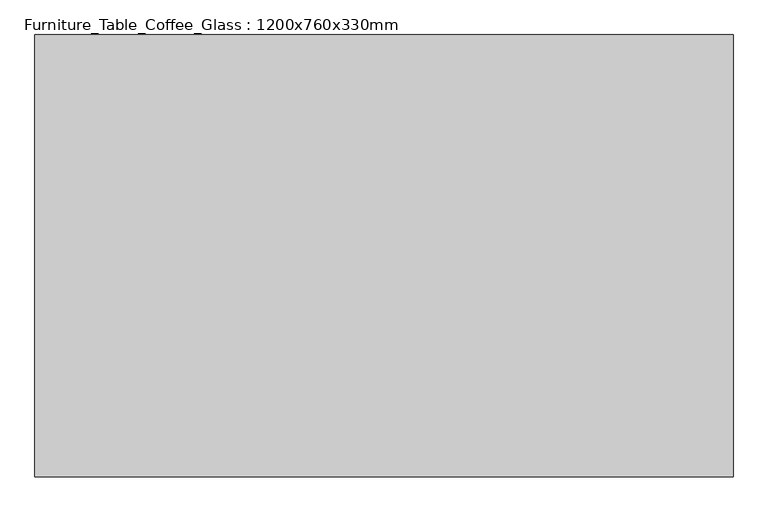
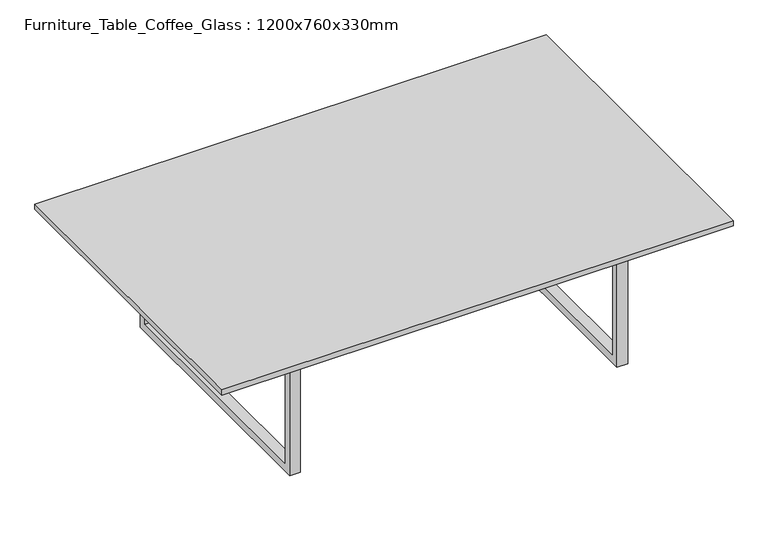
"""IFC4 building model written with IfcOpenShell, lengths in millimetres: furniture geometry, Furniture_Table_Coffee_Glass : 1200x760x330mm."""

from ifc_helpers import new_model, si_unit, frame, origin, place, context, project, spatial, polyline, outline, extrude, source, transform, mapped, element, save


def furniture_table_coffee_glass_1200x760x330mm_bccf866f(model_context):
    return source(origin(), model_context, "Body", "SweptSolid", [
        extrude(outline(polyline([(1203.7336303, 748.6108318), (1203.7336303, -11.3891682), (3.7336303, -11.3891682), (3.7336303, 748.6108318), (1203.7336303, 748.6108318)])), frame((0.0, 0.0, 317.3), z_axis=(0.0, 0.0, 1.0), x_axis=(1.0, 0.0, 0.0)), (0.0, 0.0, 1.0), 12.7),
        extrude(outline(polyline([(64.8108318, 317.3), (672.4108318, 317.3), (672.4108318, 0.0), (64.8108318, 0.0), (64.8108318, 317.3)]), holes=[polyline([(83.8608318, 298.25), (83.8608318, 19.05), (653.3608318, 19.05), (653.3608318, 298.25), (83.8608318, 298.25)])]), frame((206.9336303, 0.0, 0.0), z_axis=(1.0, 0.0, 0.0), x_axis=(0.0, 1.0, 0.0)), (0.0, 0.0, 1.0), 25.4),
        extrude(outline(polyline([(64.8108318, 317.3), (672.4108318, 317.3), (672.4108318, 0.0), (64.8108318, 0.0), (64.8108318, 317.3)]), holes=[polyline([(83.8608318, 298.25), (83.8608318, 19.05), (653.3608318, 19.05), (653.3608318, 298.25), (83.8608318, 298.25)])]), frame((975.1336303, 0.0, 0.0), z_axis=(1.0, 0.0, 0.0), x_axis=(0.0, 1.0, 0.0)), (0.0, 0.0, 1.0), 25.4),
        extrude(outline(polyline([(975.1336303, 378.1358318), (975.1336303, 359.0858318), (232.3336303, 359.0858318), (232.3336303, 378.1358318), (975.1336303, 378.1358318)])), frame((0.0, 0.0, 298.25), z_axis=(0.0, 0.0, 1.0), x_axis=(1.0, 0.0, 0.0)), (0.0, 0.0, 1.0), 19.05),
    ])


if __name__ == "__main__":
    model = new_model("IFC4")
    model_context = context("Model", 3, world=origin())
    ifc_project = project(units=[si_unit("LENGTHUNIT", "METRE", prefix="MILLI")], contexts=[model_context])
    site = spatial("IfcSite", under=ifc_project)
    building = spatial("IfcBuilding", under=site)
    placement = place(None, origin())
    furniture_table_coffee_glass_1200x760x330mm_shape = furniture_table_coffee_glass_1200x760x330mm_bccf866f(model_context)
    element("IfcFurniture", 1, ObjectType="Furniture_Table_Coffee_Glass : 1200x760x330mm", at=placement, inside=building, context=model_context, shape_type="MappedRepresentation", body=[
        mapped(furniture_table_coffee_glass_1200x760x330mm_shape, transform((0.0, 0.0, 0.0), x_axis=(1.0, 0.0, 0.0), y_axis=(0.0, 1.0, 0.0), z_axis=(0.0, 0.0, 1.0))),
    ])
    save(model, "model.ifc")

# Revit data of these elements
# Type "Furniture_Table_Coffee_Glass : 1200x760x330mm"
#   Keynote = "N"
#   Height = 1' - 0.99213"
#   Length = 3' - 11.24409"
#   Width = 2' - 5.92126"
#   Material Base = Metal - Chrome
#   Material Top = Glass - Clear, Grey
#   Default Elevation = 0
#   Assembly Code = ""
# Element 1 (IfcFurniture, "Furniture_Table_Coffee_Glass : 1200x760x330mm")
#   Materials on its faces: "Metal - Chrome", "Glass - Clear, Grey"
# Materials
#   "Metal - Chrome": class "Metal", colour RGB 17 17 17, transparency 0
#   "Glass - Clear, Grey": class "Glass", colour RGB 252 255 255, transparency 0.64
